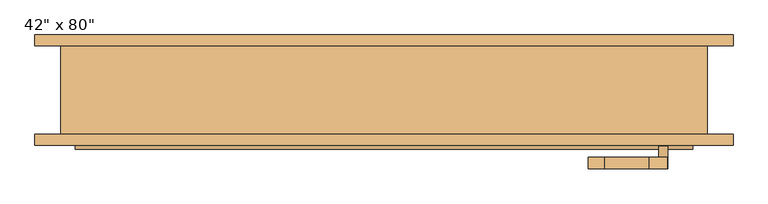
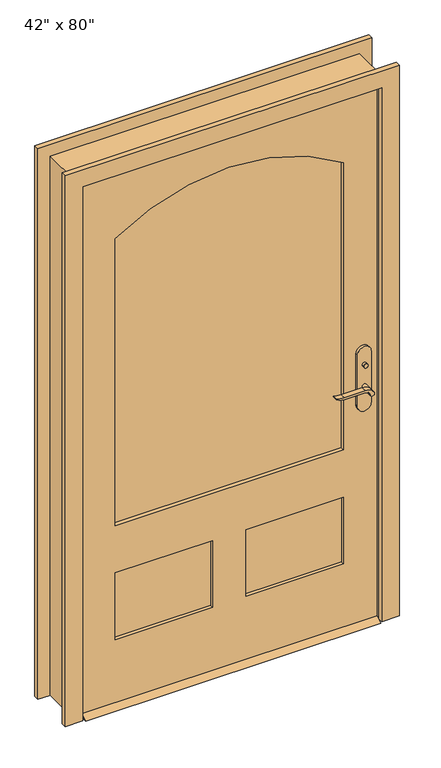
"""IFC4 building model written with IfcOpenShell, lengths in millimetres: door geometry."""

from ifc_helpers import new_model, si_unit, point, frame, frame_2d, origin, place, context, project, spatial, polyline, circle_curve, trimmed, segment, composite_curve, outline, extrude, faceted_brep, source, transform, mapped, element, save


def door_25c67de5(model_context):
    return source(origin(), model_context, "Body", "SolidModel", [
        extrude(outline(polyline([(-38.1, 12.7), (-12.7, 0.0), (-98.425, 0.0), (-73.025, 12.7), (-38.1, 12.7)])), frame((-533.4, 0.0, 0.0), z_axis=(1.0, 0.0, 0.0), x_axis=(0.0, 1.0, 0.0)), (0.0, 0.0, 1.0), 1066.8),
        extrude(outline(polyline([(487.6, -18.1), (487.6, -28.1), (477.6, -28.1), (477.6, -18.1), (487.6, -18.1)])), frame((0.0, 0.0, 981.9), z_axis=(0.0, 0.0, 1.0), x_axis=(1.0, 0.0, 0.0)), (0.0, 0.0, 1.0), 30.0),
        extrude(outline(composite_curve([segment(trimmed(circle_curve(frame_2d((996.9, 482.6)), 8.0), [point((996.9, 474.6))], [point((996.9, 490.6))], False, "CARTESIAN"), True, "CONTINUOUS"), segment(trimmed(circle_curve(frame_2d((996.9, 482.6)), 8.0), [point((996.9, 490.6))], [point((996.9, 474.6))], False, "CARTESIAN"), True, "CONTINUOUS")], self_intersect=False)), frame((0.0, -93.025, 0.0), z_axis=(0.0, 1.0, 0.0), x_axis=(0.0, 0.0, 1.0)), (0.0, 0.0, 1.0), 10.0),
        extrude(outline(composite_curve([segment(trimmed(circle_curve(frame_2d((897.1555521, 458.9324871)), 37.2832219), [point((919.0523287, 489.1081363))], [point((934.4, 457.2325667))], False, "CARTESIAN"), True, "CONTINUOUS"), segment(polyline([(934.4, 457.2325667), (934.4, 380.9564091)]), True, "CONTINUOUS"), segment(trimmed(circle_curve(frame_2d((1017.6850638, 381.0227909)), 83.2850902), [point((934.4, 380.9564091))], [point((939.4, 352.6))], True, "CARTESIAN"), True, "CONTINUOUS"), segment(polyline([(939.4, 352.6), (936.6135558, 352.6)]), True, "CONTINUOUS"), segment(trimmed(circle_curve(frame_2d((986.6709207, 384.5396612)), 59.3791355), [point((936.6135558, 352.6))], [point((927.4, 380.9564091))], False, "CARTESIAN"), True, "CONTINUOUS"), segment(polyline([(927.4, 380.9564091), (927.4, 457.2138099)]), True, "CONTINUOUS"), segment(trimmed(circle_curve(frame_2d((909.2738613, 457.2138099)), 18.1261387), [point((927.4, 457.2138099))], [point((914.4, 474.6))], True, "CARTESIAN"), True, "CONTINUOUS"), segment(trimmed(circle_curve(frame_2d((914.4, 482.6)), 8.0), [point((914.4, 474.6))], [point((919.0523287, 489.1081363))], False, "CARTESIAN"), True, "CONTINUOUS")], self_intersect=False)), frame((0.0, 1.9, 0.0), z_axis=(0.0, 1.0, 0.0), x_axis=(0.0, 0.0, 1.0)), (0.0, 0.0, 1.0), 20.0),
        extrude(outline(composite_curve([segment(trimmed(circle_curve(frame_2d((914.4, 482.6)), 8.0), [point((914.3999903, 474.6))], [point((919.0523287, 489.1081363))], False, "CARTESIAN"), True, "CONTINUOUS"), segment(trimmed(circle_curve(frame_2d((897.1555521, 458.9324871)), 37.2832219), [point((919.0523287, 489.1081363))], [point((934.4, 457.2325667))], False, "CARTESIAN"), True, "CONTINUOUS"), segment(polyline([(934.4, 457.2325667), (934.4, 380.9564091)]), True, "CONTINUOUS"), segment(trimmed(circle_curve(frame_2d((1017.6850638, 381.0227909)), 83.2850902), [point((934.4, 380.9564091))], [point((939.4, 352.6))], True, "CARTESIAN"), True, "CONTINUOUS"), segment(polyline([(939.4, 352.6), (936.6135558, 352.6)]), True, "CONTINUOUS"), segment(trimmed(circle_curve(frame_2d((986.6709207, 384.5396612)), 59.3791355), [point((936.6135558, 352.6))], [point((927.4, 380.9564091))], False, "CARTESIAN"), True, "CONTINUOUS"), segment(polyline([(927.4, 380.9564091), (927.4, 457.2138122)]), True, "CONTINUOUS"), segment(trimmed(circle_curve(frame_2d((909.2738682, 457.2138122)), 18.1261318), [point((927.4, 457.2138122))], [point((914.3999903, 474.6))], True, "CARTESIAN"), True, "CONTINUOUS")], self_intersect=False)), frame((0.0, -133.025, 0.0), z_axis=(0.0, 1.0, 0.0), x_axis=(0.0, 0.0, 1.0)), (0.0, 0.0, 1.0), 20.0),
        extrude(outline(composite_curve([segment(trimmed(circle_curve(frame_2d((914.4, 482.6)), 8.0), [point((914.4, 474.6))], [point((914.4, 490.6))], False, "CARTESIAN"), True, "CONTINUOUS"), segment(trimmed(circle_curve(frame_2d((914.4, 482.6)), 8.0), [point((914.4, 490.6))], [point((914.4, 474.6))], False, "CARTESIAN"), True, "CONTINUOUS")], self_intersect=False)), frame((0.0, -28.1, 0.0), z_axis=(0.0, 1.0, 0.0), x_axis=(0.0, 0.0, 1.0)), (0.0, 0.0, 1.0), 30.0),
        extrude(outline(composite_curve([segment(trimmed(circle_curve(frame_2d((914.4, 482.6)), 8.0), [point((914.4, 474.6))], [point((914.4, 490.6))], False, "CARTESIAN"), True, "CONTINUOUS"), segment(trimmed(circle_curve(frame_2d((914.4, 482.6)), 8.0), [point((914.4, 490.6))], [point((914.4, 474.6))], False, "CARTESIAN"), True, "CONTINUOUS")], self_intersect=False)), frame((0.0, -113.025, 0.0), z_axis=(0.0, 1.0, 0.0), x_axis=(0.0, 0.0, 1.0)), (0.0, 0.0, 1.0), 30.0),
        extrude(outline(composite_curve([segment(polyline([(844.4, 507.6), (1039.4, 507.6)]), True, "CONTINUOUS"), segment(trimmed(circle_curve(frame_2d((1039.4, 482.6)), 25.0), [point((1039.4, 507.6))], [point((1039.4, 457.6))], False, "CARTESIAN"), True, "CONTINUOUS"), segment(polyline([(1039.4, 457.6), (844.4, 457.6)]), True, "CONTINUOUS"), segment(trimmed(circle_curve(frame_2d((844.4, 482.6)), 25.0), [point((844.4, 457.6))], [point((844.4, 507.6))], False, "CARTESIAN"), True, "CONTINUOUS")], self_intersect=False)), frame((0.0, -38.1, 0.0), z_axis=(0.0, 1.0, 0.0), x_axis=(0.0, 0.0, 1.0)), (0.0, 0.0, 1.0), 10.0),
        extrude(outline(composite_curve([segment(polyline([(844.4, 507.6), (1039.4, 507.6)]), True, "CONTINUOUS"), segment(trimmed(circle_curve(frame_2d((1039.4, 482.6)), 25.0), [point((1039.4, 507.6))], [point((1039.4, 457.6))], False, "CARTESIAN"), True, "CONTINUOUS"), segment(polyline([(1039.4, 457.6), (844.4, 457.6)]), True, "CONTINUOUS"), segment(trimmed(circle_curve(frame_2d((844.4, 482.6)), 25.0), [point((844.4, 457.6))], [point((844.4, 507.6))], False, "CARTESIAN"), True, "CONTINUOUS")], self_intersect=False)), frame((0.0, -83.025, 0.0), z_axis=(0.0, 1.0, 0.0), x_axis=(0.0, 0.0, 1.0)), (0.0, 0.0, 1.0), 10.0),
        extrude(outline(polyline([(2032.0, -533.4), (12.7, -533.4), (12.7, 533.4), (2032.0, 533.4), (2032.0, -533.4)]), holes=[composite_curve([segment(polyline([(688.975, -412.75), (1784.35, -412.75)]), True, "CONTINUOUS"), segment(trimmed(circle_curve(frame_2d((1177.13125, 0.0)), 734.21875), [point((1784.35, -412.75))], [point((1784.35, 412.75))], True, "CARTESIAN"), True, "CONTINUOUS"), segment(polyline([(1784.35, 412.75), (688.975, 412.75), (688.975, -412.75)]), True, "CONTINUOUS")], self_intersect=False), polyline([(508.0, -60.325), (254.0, -60.325), (254.0, -412.75), (508.0, -412.75), (508.0, -60.325)]), polyline([(508.0, 412.75), (254.0, 412.75), (254.0, 60.325), (508.0, 60.325), (508.0, 412.75)])]), frame((0.0, -73.025, 0.0), z_axis=(0.0, 1.0, 0.0), x_axis=(0.0, 0.0, 1.0)), (0.0, 0.0, 1.0), 34.925),
        faceted_brep([(558.8, -73.025, 0.0), (533.4, -73.025, 0.0), (533.4, -38.1, 0.0), (520.7, -38.1, 0.0), (520.7, -3.175, 0.0), (533.4, -3.175, 0.0), (533.4, 79.375, 0.0), (558.8, 79.375, 0.0), (558.8, 79.375, 2057.4), (558.8, -73.025, 2057.4), (533.4, 79.375, 2032.0), (-533.4, 79.375, 2032.0), (-533.4, 79.375, 0.0), (-558.8, 79.375, 0.0), (-558.8, 79.375, 2057.4), (533.4, -3.175, 2032.0), (520.7, -3.175, 2019.3), (-520.7, -3.175, 2019.3), (-520.7, -3.175, 0.0), (-533.4, -3.175, 0.0), (-533.4, -3.175, 2032.0), (520.7, -38.1, 2019.3), (533.4, -38.1, 2032.0), (-533.4, -38.1, 2032.0), (-533.4, -38.1, 0.0), (-520.7, -38.1, 0.0), (-520.7, -38.1, 2019.3), (533.4, -73.025, 2032.0), (-558.8, -73.025, 2057.4), (-558.8, -73.025, 0.0), (-533.4, -73.025, 0.0), (-533.4, -73.025, 2032.0)], [[[0, 1, 2, 3, 4, 5, 6, 7]], [[7, 8, 9, 0]], [[6, 10, 11, 12, 13, 14, 8, 7]], [[5, 15, 10, 6]], [[4, 16, 17, 18, 19, 20, 15, 5]], [[3, 21, 16, 4]], [[2, 22, 23, 24, 25, 26, 21, 3]], [[1, 27, 22, 2]], [[0, 9, 28, 29, 30, 31, 27, 1]], [[8, 14, 28, 9]], [[15, 20, 11, 10]], [[21, 26, 17, 16]], [[27, 31, 23, 22]], [[29, 13, 12, 19, 18, 25, 24, 30]], [[14, 13, 29, 28]], [[20, 19, 12, 11]], [[26, 25, 18, 17]], [[31, 30, 24, 23]]]),
        extrude(outline(polyline([(-60.325, -49.7416667), (-60.325, -61.3833333), (-412.75, -61.3833333), (-412.75, -49.7416667), (-60.325, -49.7416667)])), frame((0.0, 0.0, 254.0), z_axis=(0.0, 0.0, 1.0), x_axis=(1.0, 0.0, 0.0)), (0.0, 0.0, 1.0), 254.0),
        extrude(outline(polyline([(412.75, -49.7416667), (412.75, -61.3833333), (60.325, -61.3833333), (60.325, -49.7416667), (412.75, -49.7416667)])), frame((0.0, 0.0, 254.0), z_axis=(0.0, 0.0, 1.0), x_axis=(1.0, 0.0, 0.0)), (0.0, 0.0, 1.0), 254.0),
        extrude(outline(composite_curve([segment(polyline([(688.975, -412.75), (688.975, 412.75), (1784.35, 412.75)]), True, "CONTINUOUS"), segment(trimmed(circle_curve(frame_2d((1177.13125, 0.0)), 734.21875), [point((1784.35, 412.75))], [point((1784.35, -412.75))], False, "CARTESIAN"), True, "CONTINUOUS"), segment(polyline([(1784.35, -412.75), (688.975, -412.75)]), True, "CONTINUOUS")], self_intersect=False)), frame((0.0, -59.055, 0.0), z_axis=(0.0, 1.0, 0.0), x_axis=(0.0, 0.0, 1.0)), (0.0, 0.0, 1.0), 6.985),
        extrude(outline(polyline([(0.0, -539.75), (2038.35, -539.75), (2038.35, 539.75), (0.0, 539.75), (0.0, 603.25), (2101.85, 603.25), (2101.85, -603.25), (0.0, -603.25), (0.0, -539.75)])), frame((0.0, 79.375, 0.0), z_axis=(0.0, 1.0, 0.0), x_axis=(0.0, 0.0, 1.0)), (0.0, 0.0, 1.0), 19.05),
        extrude(outline(polyline([(0.0, -539.75), (2038.35, -539.75), (2038.35, 539.75), (0.0, 539.75), (0.0, 603.25), (2101.85, 603.25), (2101.85, -603.25), (0.0, -603.25), (0.0, -539.75)])), frame((0.0, -92.075, 0.0), z_axis=(0.0, 1.0, 0.0), x_axis=(0.0, 0.0, 1.0)), (0.0, 0.0, 1.0), 19.05),
    ])


if __name__ == "__main__":
    model = new_model("IFC4")
    model_context = context("Model", 3, world=origin())
    ifc_project = project(units=[si_unit("LENGTHUNIT", "METRE", prefix="MILLI")], contexts=[model_context])
    site = spatial("IfcSite", under=ifc_project)
    building = spatial("IfcBuilding", under=site)
    placement = place(None, origin())
    door_shape = door_25c67de5(model_context)
    element("IfcDoor", 1, ObjectType="42\" x 80\"", at=placement, inside=building, context=model_context, shape_type="MappedRepresentation", body=[
        mapped(door_shape, transform((0.0, 0.0, 0.0), x_axis=(1.0, 0.0, 0.0), y_axis=(0.0, 1.0, 0.0), z_axis=(0.0, 0.0, 1.0))),
    ])
    save(model, "model.ifc")

# Revit data of these elements
# Type "42\" x 80\""
#   Type Mark = "8"
#   Assembly Code = "B2030100"
#   Analytic Construction = "French door, wood frame with single glass"
#   Threshold Offset [instance default] = 0' - 0 1/2"
#   Thickness = 0' - 1 3/8"
#   Thermal Resistance (R) = 1.0696 (h·ft²·°F)/BTU
#   Swing Angle [instance default] = 90.00°
#   Stiles = 0' - 4 3/4"
#   Rough Width = 3' - 8"
#   Rough Height = 6' - 9"
#   Radius = 2' - 4 29/32"
#   Lock Rail = 0' - 7 1/8"
#   Height = 6' - 8"
#   Width = 3' - 6"
#   Heat Transfer Coefficient (U) = 0.9350 BTU/(h·ft²·°F)
#   Door Offset [instance default] = 0' - 0"
#   Bottom Rail = 0' - 9 1/2"
#   Threshold [instance default] = yes
#   Function = 1
#   Exterior Trim [instance default] = yes
#   Trim Material = Cherry
#   Threshold Material = Cherry
#   Panel Material = Cherry
#   Glazing = Glass
#   Frame Material = Cherry
#   Door Handle Material = Aluminum
#   Visual Light Transmittance = 0
#   Solar Heat Gain Coefficient = 0
#   Wall Closure = (empty or 0)
#   Construction Type = (empty or 0)
# Element 1 (IfcDoor, "42\" x 80\"")
#   Materials on its faces: "Cherry", "Aluminum", "Glass"
# Materials
#   "Cherry": class "Wood", colour RGB 226 177 128, transparency 0, Description = "Prunus Serotina", Cost = 0
#   "Glass": class "Glass", colour RGB 0 128 192, transparency 0.75, Description = "Soda Lime Glass", Cost = 0
#   "Aluminum": class "Metal", colour RGB 247 247 247, transparency 0, Description = "Aluminum 6061", Cost = 0
